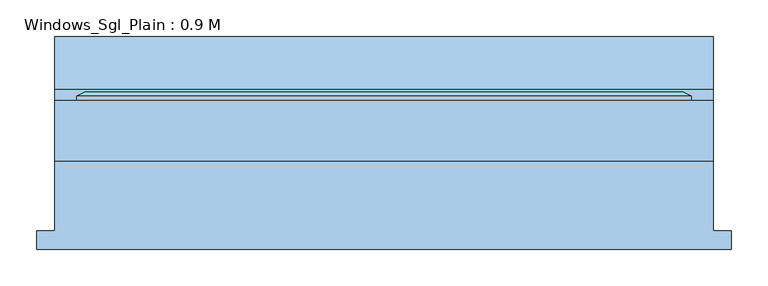
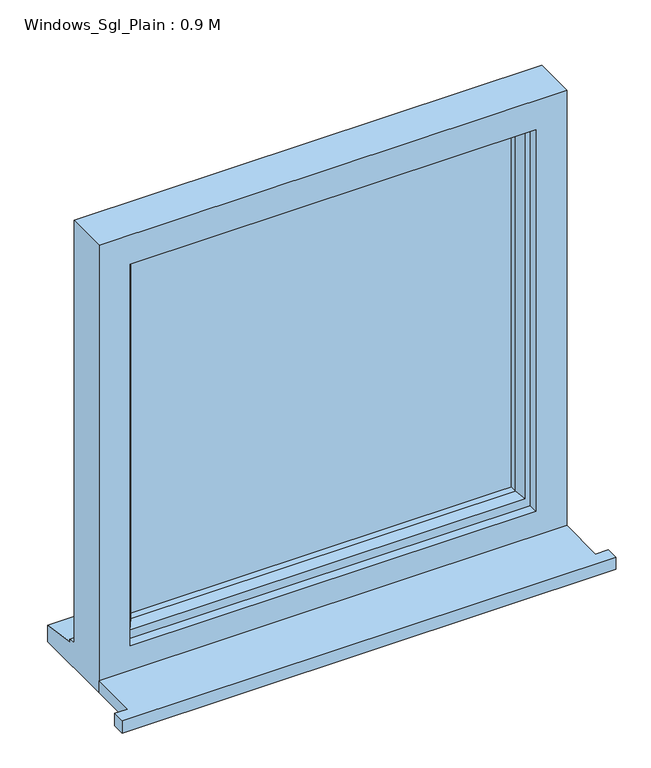
"""IFC4 building model written with IfcOpenShell, lengths in millimetres: window geometry, Windows_Sgl_Plain : 0.9 M."""

from ifc_helpers import new_model, si_unit, frame, origin, place, context, project, spatial, polyline, outline, extrude, faceted_brep, source, transform, mapped, element, save


def windows_sgl_plain_0_9_m_ad1c2cf7(model_context):
    return source(origin(), model_context, "Body", "SolidModel", [
        extrude(outline(polyline([(-475.0, -130.8434322), (-475.0, -105.8434322), (-450.0, -105.8434322), (-450.0, -10.2434322), (450.0, -10.2434322), (450.0, -105.8434322), (475.0, -105.8434322), (475.0, -130.8434322), (-475.0, -130.8434322)])), frame((0.0, 0.0, 1200.0), z_axis=(0.0, 0.0, 1.0), x_axis=(1.0, 0.0, 0.0)), (0.0, 0.0, 1.0), 25.0),
        faceted_brep([(-450.0, -10.2434322, 1200.0), (450.0, -10.2434322, 1200.0), (450.0, -10.2434322, 2110.0), (-450.0, -10.2434322, 2110.0), (-390.0, -10.2434322, 2050.0), (390.0, -10.2434322, 2050.0), (390.0, -10.2434322, 1275.0), (-390.0, -10.2434322, 1275.0), (-450.0, 72.7565678, 2110.0), (-450.0, 72.7565678, 1251.0), (-450.0, 87.7565678, 1249.68767), (-450.0, 87.7565678, 1244.7449676), (-450.0, 160.2565678, 1233.8088847), (-450.0, 160.2565678, 1200.0), (450.0, 72.7565678, 2110.0), (450.0, 72.7565678, 1251.0), (-410.0, 72.7565678, 2070.0), (-410.0, 72.7565678, 1263.0), (410.0, 72.7565678, 1263.0), (410.0, 72.7565678, 2070.0), (-410.0, 7.7565678, 2070.0), (-410.0, 7.7565678, 1263.0), (410.0, 7.7565678, 2070.0), (410.0, 7.7565678, 1263.0), (-390.0, 7.7565678, 2050.0), (-390.0, 7.7565678, 1275.0), (390.0, 7.7565678, 1275.0), (390.0, 7.7565678, 2050.0), (450.0, 160.2565678, 1200.0), (450.0, 160.2565678, 1233.8088847), (450.0, 87.7565678, 1244.7449676), (450.0, 87.7565678, 1249.68767)], [[[0, 1, 2, 3], [4, 5, 6, 7]], [[0, 3, 8, 9, 10, 11, 12, 13]], [[9, 8, 14, 15], [16, 17, 18, 19]], [[17, 16, 20, 21]], [[20, 22, 23, 21], [24, 25, 26, 27]], [[24, 4, 7, 25]], [[3, 2, 14, 8]], [[16, 19, 22, 20]], [[5, 4, 24, 27]], [[15, 14, 2, 1, 28, 29, 30, 31]], [[19, 18, 23, 22]], [[5, 27, 26, 6]], [[28, 1, 0, 13]], [[29, 28, 13, 12]], [[30, 29, 12, 11]], [[31, 30, 11, 10]], [[15, 31, 10, 9]], [[21, 23, 18, 17]], [[7, 6, 26, 25]]]),
        extrude(outline(polyline([(380.0, 36.7565678), (-380.0, 36.7565678), (-380.0, 60.7565678), (380.0, 60.7565678), (380.0, 36.7565678)])), frame((0.0, 0.0, 1293.0), z_axis=(0.0, 0.0, 1.0), x_axis=(1.0, 0.0, 0.0)), (0.0, 0.0, 1.0), 747.0),
        faceted_brep([(-420.0, 72.7565678, 2080.0), (-420.0, 78.5300705, 2080.0), (-420.0, 78.5300705, 1253.0), (-420.0, 72.7565678, 1253.0), (-410.0, 7.7565678, 2070.0), (-410.0, 72.7565678, 2070.0), (-410.0, 72.7565678, 1263.0), (-410.0, 7.7565678, 1263.0), (-370.0, 22.2494677, 2030.0), (-380.1480377, 7.7565678, 2040.1480377), (-380.1480377, 7.7565678, 1292.8519623), (-370.0, 22.2494677, 1303.0), (-370.0, 36.7565678, 2030.0), (-370.0, 36.7565678, 1303.0), (-380.0, 60.7565678, 2040.0), (-380.0, 36.7565678, 2040.0), (-380.0, 36.7565678, 1293.0), (-380.0, 60.7565678, 1293.0), (-370.0, 78.5300705, 2030.0), (-370.0, 60.7565678, 2030.0), (-370.0, 60.7565678, 1303.0), (-370.0, 78.5300705, 1303.0), (-387.4457548, 84.3035732, 2047.4457548), (-387.4457548, 84.3035732, 1285.5542452), (-409.2153903, 84.3035732, 2069.2153903), (-409.2153903, 84.3035732, 1263.7846097), (420.0, 78.5300705, 1253.0), (420.0, 72.7565678, 1253.0), (410.0, 72.7565678, 1263.0), (410.0, 7.7565678, 1263.0), (380.1480377, 7.7565678, 1292.8519623), (370.0, 22.2494677, 1303.0), (370.0, 36.7565678, 1303.0), (380.0, 36.7565678, 1293.0), (380.0, 60.7565678, 1293.0), (370.0, 60.7565678, 1303.0), (370.0, 78.5300705, 1303.0), (387.4457548, 84.3035732, 1285.5542452), (409.2153903, 84.3035732, 1263.7846097), (420.0, 78.5300705, 2080.0), (420.0, 72.7565678, 2080.0), (410.0, 72.7565678, 2070.0), (410.0, 7.7565678, 2070.0), (380.1480377, 7.7565678, 2040.1480377), (370.0, 22.2494677, 2030.0), (370.0, 36.7565678, 2030.0), (380.0, 36.7565678, 2040.0), (380.0, 60.7565678, 2040.0), (370.0, 60.7565678, 2030.0), (370.0, 78.5300705, 2030.0), (387.4457548, 84.3035732, 2047.4457548), (409.2153903, 84.3035732, 2069.2153903)], [[[0, 1, 2, 3]], [[4, 5, 6, 7]], [[8, 9, 10, 11]], [[12, 8, 11, 13]], [[14, 15, 16, 17]], [[18, 19, 20, 21]], [[22, 18, 21, 23]], [[1, 24, 25, 2]], [[3, 2, 26, 27]], [[7, 6, 28, 29]], [[11, 10, 30, 31]], [[13, 11, 31, 32]], [[17, 16, 33, 34]], [[21, 20, 35, 36]], [[23, 21, 36, 37]], [[2, 25, 38, 26]], [[27, 26, 39, 40]], [[29, 28, 41, 42]], [[31, 30, 43, 44]], [[32, 31, 44, 45]], [[34, 33, 46, 47]], [[36, 35, 48, 49]], [[37, 36, 49, 50]], [[26, 38, 51, 39]], [[40, 39, 1, 0]], [[3, 27, 40, 0], [5, 41, 28, 6]], [[42, 41, 5, 4]], [[7, 29, 42, 4], [9, 43, 30, 10]], [[44, 43, 9, 8]], [[45, 44, 8, 12]], [[15, 46, 33, 16], [13, 32, 45, 12]], [[47, 46, 15, 14]], [[17, 34, 47, 14], [19, 48, 35, 20]], [[49, 48, 19, 18]], [[50, 49, 18, 22]], [[24, 51, 38, 25], [23, 37, 50, 22]], [[39, 51, 24, 1]]]),
    ])


if __name__ == "__main__":
    model = new_model("IFC4")
    model_context = context("Model", 3, world=origin())
    ifc_project = project(units=[si_unit("LENGTHUNIT", "METRE", prefix="MILLI")], contexts=[model_context])
    site = spatial("IfcSite", under=ifc_project)
    building = spatial("IfcBuilding", under=site)
    placement = place(None, origin())
    windows_sgl_plain_0_9_m_shape = windows_sgl_plain_0_9_m_ad1c2cf7(model_context)
    element("IfcWindow", 1, ObjectType="Windows_Sgl_Plain : 0.9 M", at=placement, inside=building, context=model_context, shape_type="MappedRepresentation", body=[
        mapped(windows_sgl_plain_0_9_m_shape, transform((0.0, 0.0, 0.0), x_axis=(1.0, 0.0, 0.0), y_axis=(0.0, 1.0, 0.0), z_axis=(0.0, 0.0, 1.0))),
    ])
    save(model, "model.ifc")

# Revit data of these elements
# Type "Windows_Sgl_Plain : 0.9 M"
#   Type Mark = "59"
#   Operation = "SinglePanel"
#   Construction Type Id = "SGL"
#   Manufacturer = "Revit"
#   Keynote = "L10"
#   Analytic Construction = "Large single-glazed windows"
#   Wrap Layers (Ext) from Ext = 0.1025 m
#   Wrap Layers (Int) from Ext = 0.1775 m
#   Window Board Projection = 0.025 m
#   Window Board Extension = 0.025 m
#   Visual Light Transmittance = 0.9
#   Solar Heat Gain Coefficient = 0.86
#   Rough Width = 0.9 m
#   Rough Height = 0.91 m
#   Height = 0.91 m
#   Width = 0.9 m
#   Heat Transfer Coefficient (U) = 5.5617 W/(m²·K)
#   Glazing Thickness = 0.024 m
#   FrameOffset - External = 0.05 m
#   Frame Depth = 0.065 m
#   Default Head Height = 2.11 m
#   Cill Depth = 0.0875 m
#   Cavity Closer Width = 0.05 m
#   Cavity Closer Offset from Ext = 0.1025 m
#   Cavity Closer Depth = 0.085 m
#   Vis - Cavity Closers = yes
#   Define Thermal Properties by = 1
#   Material Trim = Window Frame
#   Material Glass = Glass
#   Material Frame = Window Frame
#   Wall Closure = (empty or 0)
# Element 1 (IfcWindow, "Windows_Sgl_Plain : 0.9 M")
#   Materials on its faces: "Window Frame", "Glass"
# Materials
#   "Window Frame": colour RGB 249 249 249, transparency 0, Keynote = "L10", Cost = 0
#   "Glass": class "Glass", colour RGB 0 128 192, transparency 0.9, Description = "Soda Lime Glass", Cost = 0
